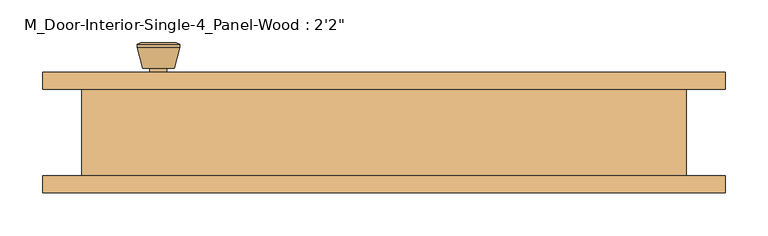
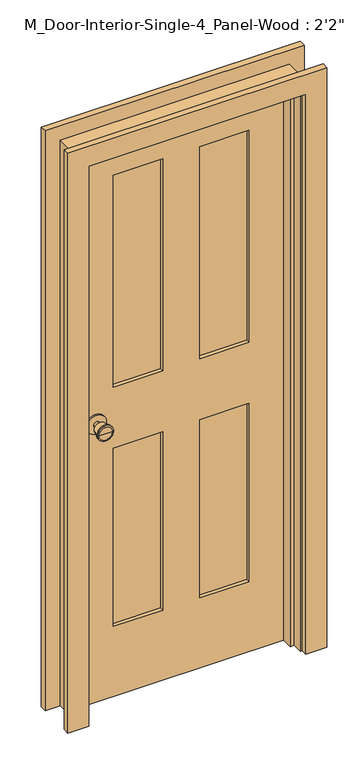
"""IFC4 building model written with IfcOpenShell, lengths in millimetres: door geometry."""

from ifc_helpers import new_model, si_unit, point, frame, frame_2d, origin, place, context, project, spatial, polyline, circle_curve, trimmed, segment, composite_curve, outline, extrude, faceted_brep, source, transform, mapped, element, save
from ifc_brep_helpers import plane_surface, cylinder_surface, revolved_surface, advanced_brep


def door_7e1124f1(model_context):
    return source(origin(), model_context, "Body", "SolidModel", [
        advanced_brep(
        [(-265.2, 6.625, 914.4), (-255.2, 6.625, 914.4), (-275.2, 6.625, 914.4), (-244.7241324, -42.375, 914.4), (-265.2, -42.375, 914.4), (-285.6758676, -42.375, 914.4), (-240.2, -40.5471319, 914.4), (-290.2, -40.5471319, 914.4), (-240.2, -37.0834537, 914.4), (-290.2, -37.0834537, 914.4), (-246.563764, -12.375, 914.4), (-283.836236, -12.375, 914.4), (-255.2, -12.375, 914.4), (-275.2, -12.375, 914.4)],
        [
            (0, 1),
            (1, 2, circle_curve(frame((-265.2, 6.625, 914.4), z_axis=(0.0, 1.0, 0.0), x_axis=(-1.0, 0.0, 0.0)), 10.0)),
            (2, 0),
            (2, 1, circle_curve(frame((-265.2, 6.625, 914.4), z_axis=(0.0, 1.0, 0.0), x_axis=(-1.0, 0.0, 0.0)), 10.0)),
            (3, 4),
            (4, 5),
            (5, 3, circle_curve(frame((-265.2, -42.375, 914.4), z_axis=(0.0, -1.0, 0.0), x_axis=(-1.0, 0.0, 0.0)), 20.4758676)),
            (3, 5, circle_curve(frame((-265.2, -42.375, 914.4), z_axis=(0.0, -1.0, 0.0), x_axis=(-1.0, 0.0, 0.0)), 20.4758676)),
            (6, 3),
            (5, 7),
            (7, 6, circle_curve(frame((-265.2, -40.5471319, 914.4), z_axis=(0.0, -1.0, 0.0), x_axis=(-1.0, 0.0, 0.0)), 25.0)),
            (6, 7, circle_curve(frame((-265.2, -40.5471319, 914.4), z_axis=(0.0, -1.0, 0.0), x_axis=(-1.0, 0.0, 0.0)), 25.0)),
            (8, 6),
            (7, 9),
            (9, 8, circle_curve(frame((-265.2, -37.0834537, 914.4), z_axis=(0.0, -1.0, 0.0), x_axis=(-1.0, 0.0, 0.0)), 25.0)),
            (8, 9, circle_curve(frame((-265.2, -37.0834537, 914.4), z_axis=(0.0, -1.0, 0.0), x_axis=(-1.0, 0.0, 0.0)), 25.0)),
            (10, 8),
            (9, 11),
            (11, 10, circle_curve(frame((-265.2, -12.375, 914.4), z_axis=(0.0, -1.0, 0.0), x_axis=(-1.0, 0.0, 0.0)), 18.636236)),
            (10, 11, circle_curve(frame((-265.2, -12.375, 914.4), z_axis=(0.0, -1.0, 0.0), x_axis=(-1.0, 0.0, 0.0)), 18.636236)),
            (12, 10),
            (11, 13),
            (13, 12, circle_curve(frame((-265.2, -12.375, 914.4), z_axis=(0.0, -1.0, 0.0), x_axis=(-1.0, 0.0, 0.0)), 10.0)),
            (12, 13, circle_curve(frame((-265.2, -12.375, 914.4), z_axis=(0.0, -1.0, 0.0), x_axis=(-1.0, 0.0, 0.0)), 10.0)),
            (1, 12),
            (13, 2),
        ],
        [
            plane_surface(frame((-265.2, 6.625, 914.4), z_axis=(0.0, 1.0, 0.0), x_axis=(-1.0, 0.0, 0.0))),
            plane_surface(frame((-265.2, -42.375, 914.4), z_axis=(0.0, -1.0, 0.0), x_axis=(-1.0, 0.0, 0.0))),
            revolved_surface(polyline([(-285.6758676, -42.375, 914.4), (-290.2, -40.5471319, 914.4)]), (-265.2, 6.625, 914.4), (0.0, 1.0, 0.0)),
            cylinder_surface(frame((-265.2, 6.625, 914.4), z_axis=(0.0, 1.0, 0.0), x_axis=(-1.0, 0.0, 0.0)), 25.0),
            revolved_surface(polyline([(-290.2, -37.0834537, 914.4), (-283.836236, -12.375, 914.4)]), (-265.2, 6.625, 914.4), (0.0, 1.0, 0.0)),
            plane_surface(frame((-265.2, -12.375, 914.4), z_axis=(0.0, 1.0, 0.0), x_axis=(-1.0, 0.0, 0.0))),
            cylinder_surface(frame((-265.2, 6.625, 914.4), z_axis=(0.0, 1.0, 0.0), x_axis=(-1.0, 0.0, 0.0)), 10.0),
        ],
        [
            (0, [[1, 2, 3]]),
            (0, [[-3, 4, -1]]),
            (1, [[5, 6, 7]]),
            (1, [[-6, -5, 8]]),
            (2, [[9, -7, 10, 11]]),
            (2, [[-10, -8, -9, 12]]),
            (3, [[13, -11, 14, 15]]),
            (3, [[-14, -12, -13, 16]]),
            (4, [[17, -15, 18, 19]]),
            (4, [[-18, -16, -17, 20]]),
            (5, [[21, -19, 22, 23]]),
            (5, [[-22, -20, -21, 24]]),
            (6, [[25, -23, 26, -2]]),
            (6, [[-26, -24, -25, -4]]),
        ],
    ),
        extrude(outline(composite_curve([segment(trimmed(circle_curve(frame_2d((914.4, -265.2)), 30.0), [point((914.4, -295.2))], [point((914.4, -235.2))], False, "CARTESIAN"), True, "CONTINUOUS"), segment(trimmed(circle_curve(frame_2d((914.4, -265.2)), 30.0), [point((914.4, -235.2))], [point((914.4, -295.2))], False, "CARTESIAN"), True, "CONTINUOUS")], self_intersect=False)), frame((0.0, 6.625, 0.0), z_axis=(0.0, 1.0, 0.0), x_axis=(0.0, 0.0, 1.0)), (0.0, 0.0, 1.0), 6.0),
        advanced_brep(
        [(-265.2, 53.625, 914.4), (-275.2, 53.625, 914.4), (-255.2, 53.625, 914.4), (-244.7241324, 102.625, 914.4), (-285.6758676, 102.625, 914.4), (-265.2, 102.625, 914.4), (-240.2, 100.7971319, 914.4), (-290.2, 100.7971319, 914.4), (-240.2, 97.3334537, 914.4), (-290.2, 97.3334537, 914.4), (-246.563764, 72.625, 914.4), (-283.836236, 72.625, 914.4), (-255.2, 72.625, 914.4), (-275.2, 72.625, 914.4)],
        [
            (0, 1),
            (1, 2, circle_curve(frame((-265.2, 53.625, 914.4), z_axis=(0.0, -1.0, 0.0), x_axis=(-1.0, 0.0, 0.0)), 10.0)),
            (2, 0),
            (2, 1, circle_curve(frame((-265.2, 53.625, 914.4), z_axis=(0.0, -1.0, 0.0), x_axis=(-1.0, 0.0, 0.0)), 10.0)),
            (3, 4, circle_curve(frame((-265.2, 102.625, 914.4), z_axis=(0.0, 1.0, 0.0), x_axis=(-1.0, 0.0, 0.0)), 20.4758676)),
            (4, 5),
            (5, 3),
            (4, 3, circle_curve(frame((-265.2, 102.625, 914.4), z_axis=(0.0, 1.0, 0.0), x_axis=(-1.0, 0.0, 0.0)), 20.4758676)),
            (6, 7, circle_curve(frame((-265.2, 100.7971319, 914.4), z_axis=(0.0, 1.0, 0.0), x_axis=(-1.0, 0.0, 0.0)), 25.0)),
            (7, 4),
            (3, 6),
            (7, 6, circle_curve(frame((-265.2, 100.7971319, 914.4), z_axis=(0.0, 1.0, 0.0), x_axis=(-1.0, 0.0, 0.0)), 25.0)),
            (8, 9, circle_curve(frame((-265.2, 97.3334537, 914.4), z_axis=(0.0, 1.0, 0.0), x_axis=(-1.0, 0.0, 0.0)), 25.0)),
            (9, 7),
            (6, 8),
            (9, 8, circle_curve(frame((-265.2, 97.3334537, 914.4), z_axis=(0.0, 1.0, 0.0), x_axis=(-1.0, 0.0, 0.0)), 25.0)),
            (10, 11, circle_curve(frame((-265.2, 72.625, 914.4), z_axis=(0.0, 1.0, 0.0), x_axis=(-1.0, 0.0, 0.0)), 18.636236)),
            (11, 9),
            (8, 10),
            (11, 10, circle_curve(frame((-265.2, 72.625, 914.4), z_axis=(0.0, 1.0, 0.0), x_axis=(-1.0, 0.0, 0.0)), 18.636236)),
            (12, 13, circle_curve(frame((-265.2, 72.625, 914.4), z_axis=(0.0, 1.0, 0.0), x_axis=(-1.0, 0.0, 0.0)), 10.0)),
            (13, 11),
            (10, 12),
            (13, 12, circle_curve(frame((-265.2, 72.625, 914.4), z_axis=(0.0, 1.0, 0.0), x_axis=(-1.0, 0.0, 0.0)), 10.0)),
            (1, 13),
            (12, 2),
        ],
        [
            plane_surface(frame((-265.2, 53.625, 914.4), z_axis=(0.0, -1.0, 0.0), x_axis=(-1.0, 0.0, 0.0))),
            plane_surface(frame((-265.2, 102.625, 914.4), z_axis=(0.0, 1.0, 0.0), x_axis=(-1.0, 0.0, 0.0))),
            revolved_surface(polyline([(-285.6758676, 102.625, 914.4), (-290.2, 100.7971319, 914.4)]), (-265.2, 53.625, 914.4), (0.0, -1.0, 0.0)),
            cylinder_surface(frame((-265.2, 53.625, 914.4), z_axis=(0.0, -1.0, 0.0), x_axis=(-1.0, 0.0, 0.0)), 25.0),
            revolved_surface(polyline([(-290.2, 97.3334537, 914.4), (-283.836236, 72.625, 914.4)]), (-265.2, 53.625, 914.4), (0.0, -1.0, 0.0)),
            plane_surface(frame((-265.2, 72.625, 914.4), z_axis=(0.0, -1.0, 0.0), x_axis=(-1.0, 0.0, 0.0))),
            cylinder_surface(frame((-265.2, 53.625, 914.4), z_axis=(0.0, -1.0, 0.0), x_axis=(-1.0, 0.0, 0.0)), 10.0),
        ],
        [
            (0, [[1, 2, 3]]),
            (0, [[-3, 4, -1]]),
            (1, [[5, 6, 7]]),
            (1, [[8, -7, -6]]),
            (2, [[9, 10, -5, 11]]),
            (2, [[12, -11, -8, -10]]),
            (3, [[13, 14, -9, 15]]),
            (3, [[16, -15, -12, -14]]),
            (4, [[17, 18, -13, 19]]),
            (4, [[20, -19, -16, -18]]),
            (5, [[21, 22, -17, 23]]),
            (5, [[24, -23, -20, -22]]),
            (6, [[-2, 25, -21, 26]]),
            (6, [[-4, -26, -24, -25]]),
        ],
    ),
        extrude(outline(composite_curve([segment(trimmed(circle_curve(frame_2d((914.4, -265.2)), 30.0), [point((914.4, -295.2))], [point((914.4, -235.2))], False, "CARTESIAN"), True, "CONTINUOUS"), segment(trimmed(circle_curve(frame_2d((914.4, -265.2)), 30.0), [point((914.4, -235.2))], [point((914.4, -295.2))], False, "CARTESIAN"), True, "CONTINUOUS")], self_intersect=False)), frame((0.0, 47.625, 0.0), z_axis=(0.0, 1.0, 0.0), x_axis=(0.0, 0.0, 1.0)), (0.0, 0.0, 1.0), 6.0),
        faceted_brep([(355.2, 47.625, 0.0), (355.2, -53.975, 0.0), (330.2, -53.975, 0.0), (330.2, -22.3, 0.0), (317.5, -22.3, 0.0), (317.5, 12.625, 0.0), (330.2, 12.625, 0.0), (330.2, 47.625, 0.0), (355.2, 47.625, 1853.8), (355.2, -53.975, 1853.8), (-355.2, -53.975, 1853.8), (-355.2, -53.975, 0.0), (-330.2, -53.975, 0.0), (-330.2, -53.975, 1828.8), (330.2, -53.975, 1828.8), (330.2, -22.3, 1828.8), (-330.2, -22.3, 1828.8), (-330.2, -22.3, 0.0), (-317.5, -22.3, 0.0), (-317.5, -22.3, 1816.1), (317.5, -22.3, 1816.1), (317.5, 12.625, 1816.1), (-317.5, 12.625, 1816.1), (-317.5, 12.625, 0.0), (-330.2, 12.625, 0.0), (-330.2, 12.625, 1828.8), (330.2, 12.625, 1828.8), (330.2, 47.625, 1828.8), (-330.2, 47.625, 1828.8), (-330.2, 47.625, 0.0), (-355.2, 47.625, 0.0), (-355.2, 47.625, 1853.8)], [[[0, 1, 2, 3, 4, 5, 6, 7]], [[1, 0, 8, 9]], [[2, 1, 9, 10, 11, 12, 13, 14]], [[3, 2, 14, 15]], [[4, 3, 15, 16, 17, 18, 19, 20]], [[5, 4, 20, 21]], [[6, 5, 21, 22, 23, 24, 25, 26]], [[7, 6, 26, 27]], [[0, 7, 27, 28, 29, 30, 31, 8]], [[9, 8, 31, 10]], [[15, 14, 13, 16]], [[21, 20, 19, 22]], [[27, 26, 25, 28]], [[30, 29, 24, 23, 18, 17, 12, 11]], [[10, 31, 30, 11]], [[16, 13, 12, 17]], [[22, 19, 18, 23]], [[28, 25, 24, 29]]]),
        extrude(outline(polyline([(1828.8, -330.2), (0.0, -330.2), (0.0, 330.2), (1828.8, 330.2), (1828.8, -330.2)]), holes=[polyline([(1708.8, 57.5), (1708.8, 210.2), (1014.4, 210.2), (1014.4, 57.5), (1708.8, 57.5)]), polyline([(1014.4, -57.5), (1014.4, -210.2), (1708.8, -210.2), (1708.8, -57.5), (1014.4, -57.5)]), polyline([(814.4, 57.5), (814.4, 210.2), (230.0, 210.2), (230.0, 57.5), (814.4, 57.5)]), polyline([(230.0, -57.5), (230.0, -210.2), (814.4, -210.2), (814.4, -57.5), (230.0, -57.5)])]), frame((0.0, 12.625, 0.0), z_axis=(0.0, 1.0, 0.0), x_axis=(0.0, 0.0, 1.0)), (0.0, 0.0, 1.0), 35.0),
        extrude(outline(polyline([(210.2, 24.2916667), (57.5, 24.2916667), (57.5, 35.9583333), (210.2, 35.9583333), (210.2, 24.2916667)])), frame((0.0, 0.0, 1014.4), z_axis=(0.0, 0.0, 1.0), x_axis=(1.0, 0.0, 0.0)), (0.0, 0.0, 1.0), 694.4),
        extrude(outline(polyline([(-57.5, 24.2916667), (-210.2, 24.2916667), (-210.2, 35.9583333), (-57.5, 35.9583333), (-57.5, 24.2916667)])), frame((0.0, 0.0, 1014.4), z_axis=(0.0, 0.0, 1.0), x_axis=(1.0, 0.0, 0.0)), (0.0, 0.0, 1.0), 694.4),
        extrude(outline(polyline([(210.2, 24.2916667), (57.5, 24.2916667), (57.5, 35.9583333), (210.2, 35.9583333), (210.2, 24.2916667)])), frame((0.0, 0.0, 230.0), z_axis=(0.0, 0.0, 1.0), x_axis=(1.0, 0.0, 0.0)), (0.0, 0.0, 1.0), 584.4),
        extrude(outline(polyline([(-57.5, 24.2916667), (-210.2, 24.2916667), (-210.2, 35.9583333), (-57.5, 35.9583333), (-57.5, 24.2916667)])), frame((0.0, 0.0, 230.0), z_axis=(0.0, 0.0, 1.0), x_axis=(1.0, 0.0, 0.0)), (0.0, 0.0, 1.0), 584.4),
        extrude(outline(polyline([(0.0, 336.55), (0.0, 401.55), (1900.15, 401.55), (1900.15, -401.55), (0.0, -401.55), (0.0, -336.55), (1835.15, -336.55), (1835.15, 336.55), (0.0, 336.55)])), frame((0.0, 47.625, 0.0), z_axis=(0.0, 1.0, 0.0), x_axis=(0.0, 0.0, 1.0)), (0.0, 0.0, 1.0), 20.0),
        extrude(outline(polyline([(0.0, 336.55), (0.0, 401.55), (1900.15, 401.55), (1900.15, -401.55), (0.0, -401.55), (0.0, -336.55), (1835.15, -336.55), (1835.15, 336.55), (0.0, 336.55)])), frame((0.0, -73.975, 0.0), z_axis=(0.0, 1.0, 0.0), x_axis=(0.0, 0.0, 1.0)), (0.0, 0.0, 1.0), 20.0),
    ])


if __name__ == "__main__":
    model = new_model("IFC4")
    model_context = context("Model", 3, world=origin())
    ifc_project = project(units=[si_unit("LENGTHUNIT", "METRE", prefix="MILLI")], contexts=[model_context])
    site = spatial("IfcSite", under=ifc_project)
    building = spatial("IfcBuilding", under=site)
    placement = place(None, origin())
    door_shape = door_7e1124f1(model_context)
    element("IfcDoor", 1, ObjectType="M_Door-Interior-Single-4_Panel-Wood : 2'2\"", at=placement, inside=building, context=model_context, shape_type="MappedRepresentation", body=[
        mapped(door_shape, transform((0.0, 0.0, 0.0), x_axis=(1.0, 0.0, 0.0), y_axis=(0.0, 1.0, 0.0), z_axis=(0.0, 0.0, 1.0))),
    ])
    save(model, "model.ifc")

# Revit data of these elements
# Type "M_Door-Interior-Single-4_Panel-Wood : 2'2\""
#   Type Mark = "43"
#   Assembly Code = "C1020300"
#   Analytic Construction = "Wooden"
#   Top Rail = 0' - 4.72441"
#   Thickness = 0' - 1.37795"
#   Thermal Resistance (R) = 0.455703 (m²·K)/W
#   Swing Angle [instance default] = 90.00°
#   Stiles = 0' - 4.72441"
#   Rough Width = 2' - 3.9685"
#   Rough Height = 6' - 0.98425"
#   Mullion = 0' - 4.52756"
#   Lock Rail = 0' - 7.87402"
#   Height = 6' - 0"
#   Width = 2' - 2"
#   Heat Transfer Coefficient (U) = 2.19465 W/(m²·K)
#   Bottom Rail = 0' - 9.05512"
#   Trim Material = Cherry
#   Panel Material = Cherry
#   Frame Material = Cherry
#   Door Handle Material = Aluminum
#   Visual Light Transmittance = 0
#   Solar Heat Gain Coefficient = 0
#   Wall Closure = (empty or 0)
#   Function = (empty or 0)
# Element 1 (IfcDoor, "M_Door-Interior-Single-4_Panel-Wood : 2'2\"")
#   Materials on its faces: "Cherry", "Aluminum"
# Materials
#   "Cherry": class "Wood", colour RGB 226 177 128, transparency 0, Description = "Prunus Serotina", Cost = 0
#   "Aluminum": class "Metal", colour RGB 247 247 247, transparency 0, Description = "Aluminum 6061", Cost = 0
